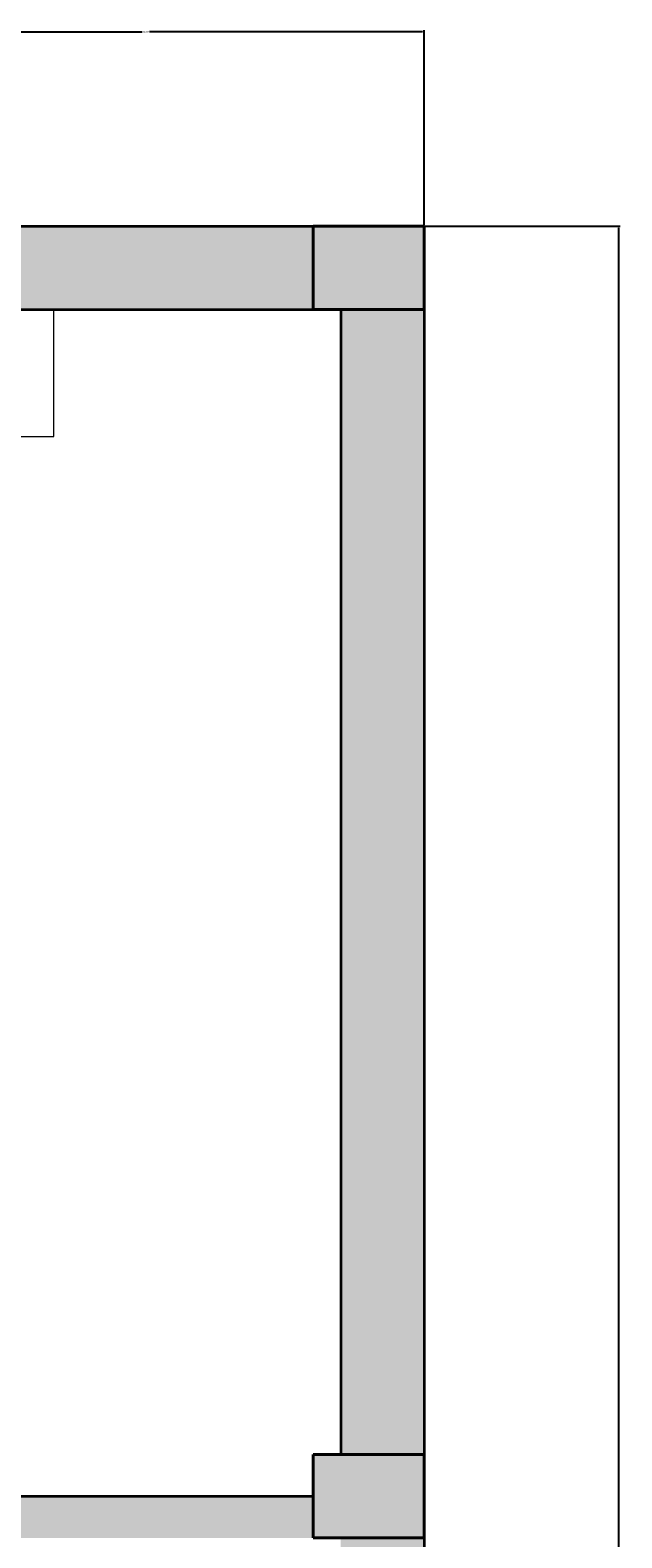
# Model space of a CAD drawing. Units: inches. Extents: x 1623 to 2200, y 2019 to 3010.
# Tile 5 of 6: x 2029 to 2093, y 2342 to 2505. Entities that reach past the tile are written whole.
import ezdxf

# ---------------------------------------------------------------- set-up
doc = ezdxf.new("R2010")
doc.units = ezdxf.units.IN
for name, color, linetype, lineweight in [('A-ANNO-DIMS', 2, 'Continuous', 18), ('A-COLS', 7, 'Continuous', 40), ('A-FURN', 8, 'Continuous', 13), ('A-WALL', 7, 'Continuous', 35)]:
    doc.layers.add(name, color=color, linetype=linetype, lineweight=lineweight)
doc.layers.add('A-COLS-PATT', color=152, linetype='Continuous', lineweight=13, true_color=0x2776bb)
doc.layers.add('A-WALL-PATT', color=251, linetype='Continuous', lineweight=13, true_color=0x636466)
doc.styles.get("Standard").update_dxf_attribs({"font": 'arial.ttf'})
doc.dimstyles.get("Standard").update_dxf_attribs({"dimtxt": 0.18, "dimasz": 0.18, "dimexe": 0.18, "dimexo": 0.0625, "dimgap": 0.09, "dimtad": 0, "dimtih": 1, "dimtoh": 1, "dimdec": 4, "dimzin": 0, "dimdsep": 46, "dimtxsty": 'Standard', "dimcen": 0.09, "dimadec": 0, "dimazin": 0, "dimtfac": 1, "dimtdec": 4, "dimtofl": 0, "dimtmove": 0, "dimatfit": 3, "dimfxl": 1, "dimtolj": 1, "dimtzin": 0, "dimarcsym": 0})

# ---------------------------------------------------------------- blocks, each defined once
blk = doc.blocks.new('COL-12X9-PLAN')
for p, q in [((0, 0), (0, 9)), ((0, 9), (12, 9)), ((12, 9), (12, 0)), ((9, 0), (0, 0)), ((12, 0), (9, 0))]:
    blk.add_line(p, q)
blk = doc.blocks.new('*D29')
at = {"layer": 'A-ANNO-DIMS', "color": 0, "lineweight": -2, "transparency": 16777216}
for p, q in [((2071.39, 2483.53), (2092.46, 2483.53)), ((2092.28, 2483.35), (2092.28, 2301.39)), ((2092.28, 2119.07), (2092.28, 2301.03)), ((2071.39, 2118.89), (2092.46, 2118.89))]:
    blk.add_line(p, q, dxfattribs=at)
at = {"layer": 'A-ANNO-DIMS', "color": 0, "transparency": 16777216}
for points in [[(2092.25, 2483.35), (2092.31, 2483.35), (2092.28, 2483.53)], [(2092.25, 2119.07), (2092.31, 2119.07), (2092.28, 2118.89)]]:
    blk.add_solid(points, dxfattribs=at)
at = {"layer": 'Defpoints', "color": 0, "transparency": 16777216}
for p in [(2071.33, 2483.53), (2092.28, 2483.53), (2071.33, 2118.89)]:
    blk.add_point(p, dxfattribs=at)
at = {"layer": 'A-ANNO-DIMS', "color": 0, "transparency": 16777216, "insert": (2092.28, 2301.21), "char_height": 0.18, "attachment_point": 5}
blk.add_mtext('\\A1;364.64', dxfattribs=at)
blk = doc.blocks.new('*D36')
at = {"layer": 'A-ANNO-DIMS', "color": 0, "lineweight": -2, "transparency": 16777216}
for p, q in [((2011.26, 2483.59), (2011.26, 2504.66)), ((2071.33, 2483.59), (2071.33, 2504.66)), ((2011.44, 2504.48), (2040.9, 2504.48)), ((2071.15, 2504.48), (2041.69, 2504.48))]:
    blk.add_line(p, q, dxfattribs=at)
at = {"layer": 'A-ANNO-DIMS', "color": 0, "transparency": 16777216}
for points in [[(2011.44, 2504.51), (2011.44, 2504.45), (2011.26, 2504.48)], [(2071.15, 2504.51), (2071.15, 2504.45), (2071.33, 2504.48)]]:
    blk.add_solid(points, dxfattribs=at)
at = {"layer": 'Defpoints', "color": 0, "transparency": 16777216}
for p in [(2071.33, 2504.48), (2011.26, 2483.52), (2071.33, 2483.53)]:
    blk.add_point(p, dxfattribs=at)
at = {"layer": 'A-ANNO-DIMS', "color": 0, "transparency": 16777216, "insert": (2041.29, 2504.48), "char_height": 0.18, "attachment_point": 5}
blk.add_mtext('\\A1;60.07', dxfattribs=at)

msp = doc.modelspace()

# ---------------------------------------------------------------- hatches: boundary and pattern name
at = {"layer": 'A-COLS-PATT'}
h = msp.add_hatch(color=256, dxfattribs=at)
h.dxf.hatch_style = 1
h.paths.add_polyline_path([(1722.3258, 2483.5237), (1710.3258, 2483.5237), (1710.3258, 2474.5237), (1719.3258, 2474.5237), (1722.3258, 2474.5237)])
h.paths.add_polyline_path([(1809.3258, 2483.5237), (1797.3258, 2483.5237), (1797.3258, 2474.5237), (1806.3258, 2474.5237), (1809.3258, 2474.5237)])
h.paths.add_polyline_path([(1918.3972, 2483.5237), (1906.3972, 2483.5237), (1906.3972, 2474.5237), (1915.3972, 2474.5237), (1918.3972, 2474.5237)])
h.paths.add_polyline_path([(2071.3258, 2483.5237), (2059.3258, 2483.5237), (2059.3258, 2474.532), (2068.3258, 2474.532), (2071.3258, 2474.532)])
h.paths.add_polyline_path([(2071.3258, 2351.0312), (2059.3258, 2351.0312), (2059.3258, 2342.0312), (2068.3258, 2342.0312), (2071.3258, 2342.0312)])
h.paths.add_polyline_path([(1918.3258, 2351.0237), (1906.3258, 2351.0237), (1906.3258, 2342.0237), (1915.3258, 2342.0237), (1918.3258, 2342.0237)])
h.paths.add_polyline_path([(1722.3198, 2351.0237), (1710.3258, 2351.0237), (1710.3258, 2342.0237), (1719.3198, 2342.0237), (1722.3198, 2342.0237)])
h.paths.add_polyline_path([(1809.3158, 2351.0237), (1797.3258, 2351.0237), (1797.3258, 2346.5237), (1797.3158, 2342.0237), (1806.3158, 2342.0237), (1809.3158, 2342.0237)])
h.paths.add_polyline_path([(1722.3029, 2170.0237), (1710.3258, 2170.0237), (1710.3258, 2161.0237), (1714.3029, 2161.0237), (1719.3029, 2161.0237), (1722.3029, 2161.0237)])
h.paths.add_polyline_path([(1809.3258, 2170.0237), (1797.3258, 2170.0237), (1797.3258, 2161.0237), (1801.3258, 2161.0237), (1802.9141, 2161.0237), (1806.3258, 2161.0237), (1809.3258, 2161.0237)])
h.paths.add_polyline_path([(1918.2273, 2170.0237), (1906.2273, 2170.0237), (1906.2273, 2161.0237), (1915.2273, 2161.0237), (1918.2273, 2161.0237)])
h.paths.add_polyline_path([(2071.3258, 2170.0237), (2059.3258, 2170.0237), (2059.3258, 2161.0237), (2068.3258, 2161.0237), (2071.3258, 2161.0237)])
at = {"layer": 'A-WALL-PATT'}
h = msp.add_hatch(color=256, dxfattribs=at)
h.dxf.hatch_style = 1
h.paths.add_polyline_path([(1725.9857, 2483.5237), (1722.3258, 2483.5237), (1722.3258, 2474.5237), (1725.9857, 2474.5237), (1725.9857, 2479.0237)])
h.paths.add_polyline_path([(1797.3258, 2483.5237), (1749.9857, 2483.5237), (1749.9857, 2474.5237), (1797.3258, 2474.5237)])
h.paths.add_polyline_path([(1830.4977, 2483.5237), (1809.3258, 2483.5237), (1809.3258, 2474.5237), (1830.4977, 2474.5237), (1830.4977, 2479.0237)])
h.paths.add_polyline_path([(1906.3972, 2483.5237), (1878.4977, 2483.5237), (1878.4977, 2474.5237), (1906.3972, 2474.5237)])
h.paths.add_polyline_path([(1918.3258, 2474.5237), (1915.3972, 2474.5237), (1913.8258, 2474.5237), (1913.8258, 2395.0237), (1913.8258, 2384.7587), (1918.3258, 2384.7587), (1918.3258, 2395.0237)])
h.paths.add_polyline_path([(1801.8258, 2474.5237), (1797.3258, 2474.5237), (1797.3258, 2436.0951), (1801.8258, 2436.0951)], flags=17)
h.paths.add_polyline_path([(1719.3258, 2474.5237), (1710.3258, 2474.5237), (1710.3258, 2351.0237), (1719.3258, 2351.0237), (1719.3258, 2395.0237), (1801.8258, 2395.0237), (1801.8258, 2399.5237), (1719.3258, 2399.5237)])
h.paths.add_polyline_path([(1797.3158, 2346.5237), (1722.3198, 2346.5237), (1722.3198, 2342.0237), (1797.3158, 2342.0237)])
h.paths.add_polyline_path([(1801.8258, 2361.4421), (1797.3258, 2361.4421), (1797.3258, 2351.0237), (1801.8258, 2351.0237)], flags=17)
h.paths.add_polyline_path([(2059.3258, 2346.5237), (1918.3258, 2346.5237), (1918.3258, 2342.0237), (2059.3258, 2342.0237)])
h.paths.add_polyline_path([(1963.26, 2479.0237), (1963.26, 2483.5237), (1918.3972, 2483.5237), (1918.3972, 2474.5237), (1963.26, 2474.5237)])
h.paths.add_polyline_path([(2059.3258, 2483.5237), (2011.26, 2483.5237), (2011.26, 2474.5237), (2059.3258, 2474.5237)])
h.paths.add_polyline_path([(2071.3258, 2474.532), (2068.3258, 2474.532), (2062.3258, 2474.532), (2062.3258, 2351.0312), (2071.3258, 2351.0312)])
h.paths.add_polyline_path([(2071.3258, 2342.0312), (2068.3258, 2342.0312), (2062.3258, 2342.0312), (2062.3258, 2170.0237), (2071.3258, 2170.0237)])
h.paths.add_polyline_path([(2059.3258, 2170.0237), (2038.3258, 2170.0237), (2038.3258, 2161.0237), (2059.3258, 2161.0237)])
h.paths.add_polyline_path([(1990.3258, 2170.0237), (1963.4402, 2170.0237), (1963.4402, 2161.0237), (1990.3258, 2161.0237), (1990.3258, 2165.5237)])
h.paths.add_polyline_path([(1918.3258, 2274.595), (1913.8258, 2274.595), (1913.8258, 2170.0237), (1918.3258, 2170.0237)])
h.paths.add_polyline_path([(1906.2273, 2170.0237), (1871.454, 2170.0237), (1871.454, 2161.0237), (1906.2273, 2161.0237)])
h.paths.add_polyline_path([(1835.454, 2170.0237), (1809.3258, 2170.0237), (1809.3258, 2161.0237), (1835.454, 2161.0237), (1835.454, 2165.5237)])
h.paths.add_polyline_path([(1801.8258, 2270.095), (1865.2406, 2270.095), (1865.2406, 2274.595), (1797.3258, 2274.595), (1797.3258, 2170.0237), (1801.8258, 2170.0237)])
h.paths.add_polyline_path([(1719.3258, 2342.0237), (1719.3198, 2342.0237), (1710.3258, 2342.0237), (1710.3258, 2170.0237), (1719.3258, 2170.0237)])

# ---------------------------------------------------------------- linework, layer by layer
at = {"layer": 'A-FURN'}
msp.add_line((2031.3673, 2474.5237), (1949.2842, 2474.5237), dxfattribs=at)
msp.add_lwpolyline([(2014.9507, 2474.5237), (2014.9507, 2460.8432), (2031.3673, 2460.8432), (2031.3673, 2474.5237)], dxfattribs=at)
at = {"layer": 'A-WALL'}
for p, q in [((1710.3258, 2483.5237), (2071.3258, 2483.5237)), ((2071.3258, 2483.5237), (2071.3258, 2161.0237)), ((1918.3258, 2474.5237), (2062.3258, 2474.5237)), ((2062.3258, 2474.5237), (2062.3258, 2351.0312)), ((1918.3258, 2346.5237), (2059.3258, 2346.5237))]:
    msp.add_line(p, q, dxfattribs=at)

# ---------------------------------------------------------------- block references
at = {"layer": 'A-COLS'}
for p in [(2059.326, 2474.5323), (2059.326, 2342.0316)]:
    msp.add_blockref('COL-12X9-PLAN', p, dxfattribs=at)

# ---------------------------------------------------------------- dimensions: what is measured, and where the dimension line sits
at = {"layer": 'A-ANNO-DIMS'}
dim = msp.add_linear_dim(base=(2071.3258, 2504.482), p1=(2011.26, 2483.5237), p2=(2071.3258, 2483.532), dimstyle='Standard', override={"dimdec": 2, "dimlfac": 1, "dimrnd": 0, "dimzin": 0, "dimdsep": 46, "dimlunit": 2}, dxfattribs=at)
dim.commit()
dim.dimension.update_dxf_attribs({"geometry": '*D36', "text_midpoint": (2041.2929, 2504.482)})
dim = msp.add_linear_dim(base=(2092.2758, 2483.532), p1=(2071.3258, 2118.8921), p2=(2071.3258, 2483.532), angle=90, dimstyle='Standard', override={"dimdec": 2, "dimlfac": 1, "dimrnd": 0, "dimzin": 0, "dimdsep": 46, "dimlunit": 2}, dxfattribs=at)
dim.commit()
dim.dimension.update_dxf_attribs({"geometry": '*D29', "text_midpoint": (2092.2758, 2301.212)})

doc.saveas('drawing.dxf')
